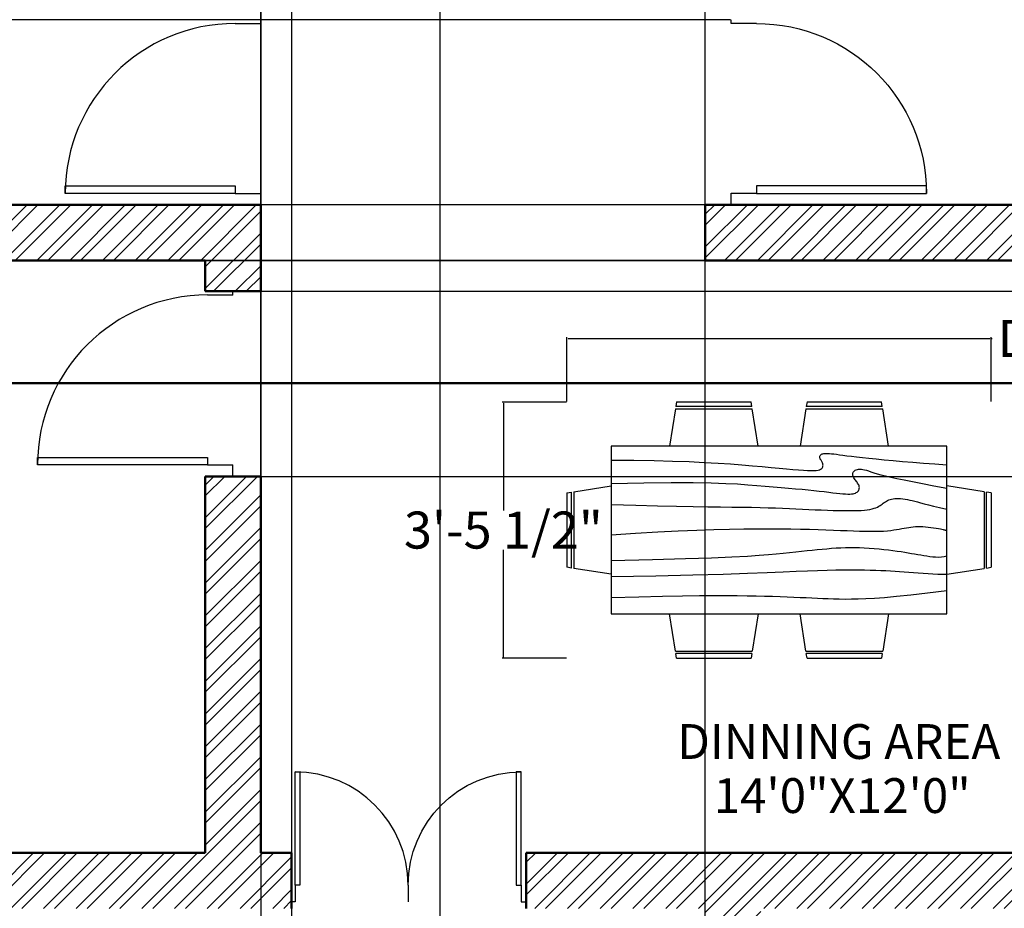
# Model space of a CAD drawing. Units: inches. Extents: x -71 to 434, y -519 to 67.
# Tile 5 of 7: x 110 to 270, y -224 to -80. Entities that reach past the tile are written whole.
import ezdxf

# ---------------------------------------------------------------- set-up
doc = ezdxf.new("R2010")
doc.units = ezdxf.units.IN
doc.header["$MEASUREMENT"] = 0
for name, color, linetype, lineweight in [('A-ANNO-DIMS', 7, 'Continuous', 18), ('A-AREA-IDEN', 7, 'Continuous', 25), ('A-WALL-PATT', 8, 'Continuous', 13), ('DOOR', 3, 'Continuous', 25), ('FURNITURE', 5, 'Continuous', 18), ('WALL', 50, 'Continuous', 50)]:
    doc.layers.add(name, color=color, linetype=linetype, lineweight=lineweight)
doc.layers.add('HATCH', color=8, linetype='Continuous')
doc.layers.add('NOI THAT', color=42, linetype='Continuous')
doc.styles.get("Standard").update_dxf_attribs({"font": 'arial.ttf'})
doc.dimstyles.get("Standard").update_dxf_attribs({"dimtxt": 6, "dimasz": 0.18, "dimexe": 0.18, "dimexo": 0.0625, "dimgap": 0.09, "dimtad": 0, "dimtih": 1, "dimtoh": 1, "dimdec": 0, "dimzin": 0, "dimdsep": 46, "dimlunit": 3, "dimtxsty": 'Standard', "dimcen": 0.09, "dimadec": 0, "dimazin": 0, "dimtfac": 1, "dimtdec": 0, "dimtofl": 0, "dimtmove": 0, "dimatfit": 3, "dimfxl": 1, "dimtolj": 1, "dimtzin": 0, "dimarcsym": 0})

# ---------------------------------------------------------------- blocks, each defined once
blk = doc.blocks.new('A$C78170A85')
at = {"layer": 'HATCH'}
for points in [[(171.5, 767.4), (258.6, 767), (337.5, 765.8), (408.9, 764), (473.5, 761.7), (532, 759), (585.1, 755.9), (633.5, 752.7), (677.8, 749.3), (718.8, 745.9), (756.5, 742.6), (790.9, 739.5), (822.2, 736.5), (850.3, 733.8), (875.4, 731.5), (897.3, 729.6), (916.3, 728.2), (932.4, 727.4), (945.8, 727.1), (956.7, 727.2), (965.6, 727.9), (972.6, 728.9), (978.1, 730.4), (982.3, 732.1), (985.5, 734.3), (988, 736.6), (989.8, 739.3), (991.1, 742.1), (991.7, 745), (991.9, 748), (991.7, 751), (991, 753.9), (990, 756.8), (988.8, 759.6), (987.3, 762.2), (985.8, 764.7), (984.2, 767.2), (982.7, 769.5), (981.4, 771.9), (980.3, 774.1), (979.5, 776.4), (979.2, 778.6), (979.2, 780.9), (979.7, 783), (980.6, 785), (982, 786.9), (983.7, 788.7), (985.9, 790.2), (988.5, 791.4), (991.6, 792.4), (995.2, 793.1), (999.4, 793.6), (1004.3, 793.7), (1010.1, 793.6), (1016.9, 793.1), (1024.7, 792.4), (1033.7, 791.4), (1043.9, 790.2), (1055.7, 788.6), (1069.2, 786.9), (1084.6, 784.9), (1102.1, 782.6), (1122, 780.2), (1144.5, 777.6), (1169.9, 774.9), (1198.1, 772), (1229.4, 769), (1263.4, 765.9), (1300.1, 762.7), (1339.4, 759.4), (1381.1, 756.1), (1425.2, 752.7), (1471.5, 749.3)], [(171.5, 677.1), (298.3, 679.7), (403.1, 680.8), (488.9, 680.7), (558.5, 679.5), (615, 677.6), (661.2, 675.2), (700.3, 672.4), (735, 669.6), (767.9, 666.8), (799.4, 664.2), (829.5, 661.7), (858.1, 659.2), (885.2, 656.9), (910.7, 654.5), (934.7, 652.3), (956.9, 650), (977.5, 647.8), (996.5, 645.6), (1013.9, 643.5), (1029.7, 641.5), (1044.1, 639.8), (1057, 638.4), (1068.6, 637.2), (1078.8, 636.5), (1087.8, 636.1), (1095.6, 636.2), (1102.4, 636.6), (1108.2, 637.4), (1113.1, 638.6), (1117.3, 640.1), (1120.9, 641.9), (1124, 644), (1126.6, 646.4), (1128.7, 649), (1130.4, 651.9), (1131.7, 654.9), (1132.4, 658.1), (1132.6, 661.3), (1132.3, 664.7), (1131.5, 668.1), (1130.1, 671.4), (1128.2, 674.8), (1126, 678.2), (1123.6, 681.6), (1121, 685), (1118.4, 688.4), (1115.8, 691.8), (1113.4, 695.1), (1111.3, 698.5), (1109.5, 701.9), (1108.2, 705.2), (1107.2, 708.5), (1106.8, 711.7), (1106.9, 714.8), (1107.6, 717.8), (1108.9, 720.7), (1110.9, 723.5), (1113.6, 726), (1116.9, 728.2), (1120.8, 730.1), (1125.1, 731.6), (1129.9, 732.6), (1135, 733), (1140.5, 732.8), (1146.3, 731.8), (1152.7, 730.3), (1159.9, 728.2), (1168.1, 725.5), (1177.6, 722.4), (1188.6, 718.9), (1201.5, 715.1), (1216.5, 710.9), (1233.8, 706.6), (1254.1, 701.9), (1277.9, 696.7), (1305.9, 690.9), (1338.7, 684.4), (1376.8, 677), (1420.9, 668.6), (1471.5, 659)], [(171.5, 595.8), (266.9, 592.9), (350.8, 590.6), (424.4, 588.9), (488.8, 587.7), (545.3, 586.9), (594.9, 586.3), (639, 585.8), (678.6, 585.3), (714.8, 584.7), (748.2, 583.9), (779.2, 583.1), (808.2, 582.1), (835.5, 581.1), (861.6, 580), (886.9, 578.9), (911.8, 577.8), (936.6, 576.7), (961.2, 575.6), (985.3, 574.6), (1008.9, 573.6), (1031.5, 572.9), (1053.1, 572.3), (1073.5, 571.9), (1092.4, 571.8), (1109.6, 571.9), (1125.2, 572.3), (1139.3, 573), (1152, 574), (1163.3, 575.3), (1173.4, 576.8), (1182.3, 578.7), (1190.2, 580.8), (1197, 583.2), (1203, 585.8), (1208.4, 588.6), (1213.1, 591.5), (1217.4, 594.5), (1221.5, 597.5), (1225.4, 600.5), (1229.3, 603.4), (1233.3, 606.1), (1237.5, 608.7), (1242, 611), (1246.8, 613.1), (1251.9, 615), (1257.4, 616.5), (1263.4, 617.6), (1269.9, 618.4), (1277, 618.8), (1284.5, 618.7), (1292.5, 618.3), (1300.9, 617.5), (1309.7, 616.3), (1318.8, 614.8), (1328.1, 613), (1337.6, 610.9), (1347.4, 608.5), (1357.9, 605.7), (1369.8, 602.5), (1383.7, 598.8), (1400.2, 594.6), (1419.9, 589.7), (1443.5, 584.1), (1471.5, 577.8)], [(171.5, 478.5), (265.6, 484.6), (351.7, 489.6), (430.6, 493.6), (502.7, 496.6), (568.7, 498.8), (629.2, 500.4), (684.7, 501.3), (735.8, 501.8), (783, 501.9), (826.7, 501.7), (867.2, 501.3), (904.8, 500.6), (939.8, 499.7), (972.5, 498.7), (1003.2, 497.6), (1032.2, 496.5), (1059.7, 495.4), (1085.8, 494.3), (1110.4, 493.4), (1133.6, 492.6), (1155.2, 492), (1175.4, 491.7), (1194.1, 491.7), (1211.2, 492), (1226.8, 492.8), (1241.1, 493.9), (1254, 495.3), (1266, 496.9), (1277, 498.7), (1287.2, 500.5), (1296.8, 502.3), (1306, 504.1), (1314.9, 505.7), (1323.7, 507.1), (1332.3, 508.3), (1341, 509.3), (1349.8, 510), (1358.9, 510.4), (1368.3, 510.4), (1378.2, 510.1), (1388.6, 509.3), (1399.3, 508.2), (1409.9, 506.9), (1420.3, 505.4), (1430, 503.8), (1438.9, 502.2), (1446.5, 500.8), (1452.7, 499.5), (1457.3, 498.5), (1460.4, 497.8), (1462.6, 497.3), (1464.1, 496.9), (1465.4, 496.7), (1466.8, 496.6), (1468.7, 496.5), (1471.5, 496.5)], [(171.5, 379.2), (330.7, 382.5), (458.9, 385.9), (560.3, 389.2), (639, 392.5), (699.2, 395.7), (745, 398.8), (780.7, 401.9), (810.2, 404.7), (837.3, 407.5), (862.5, 410.1), (886.3, 412.6), (908.7, 414.9), (929.9, 417.1), (950.2, 419.1), (969.7, 421), (988.5, 422.8), (1007, 424.4), (1025.1, 425.9), (1043, 427.1), (1060.8, 428.1), (1078.6, 428.8), (1096.5, 429.1), (1114.6, 429.2), (1133, 428.8), (1151.8, 428.1), (1170.8, 426.9), (1189.9, 425.5), (1208.8, 423.7), (1227.3, 421.8), (1245.3, 419.7), (1262.6, 417.5), (1278.9, 415.3), (1294.2, 413), (1308.5, 410.8), (1321.9, 408.5), (1334.7, 406.3), (1346.9, 404.2), (1358.8, 402.1), (1370.4, 400), (1382, 398), (1393.6, 396.1), (1405.2, 394.4), (1416.7, 393), (1428.2, 392.2), (1439.4, 392.1), (1450.5, 392.8), (1461.2, 394.4), (1471.5, 397.2)], [(171.5, 316), (344.8, 319.3), (488.1, 322.7), (605.2, 325.9), (699.8, 328.9), (776, 331.8), (837.4, 334.4), (887.9, 336.6), (931.4, 338.5), (971, 340), (1007.5, 341.1), (1041.3, 341.9), (1072.4, 342.3), (1101.2, 342.5), (1127.7, 342.4), (1152.3, 342), (1175.1, 341.6), (1196.4, 340.9), (1216.4, 340.2), (1235.3, 339.3), (1253.5, 338.3), (1271.3, 337.2), (1288.7, 335.9), (1306.3, 334.6), (1324.1, 333.3), (1342.4, 331.8), (1361.1, 330.4), (1380, 329), (1398.9, 327.7), (1417.7, 326.6), (1436.2, 325.8), (1454.2, 325.2), (1471.5, 325)], [(171.5, 234.7), (278.3, 237.7), (369.5, 239.9), (447.2, 241.5), (513.2, 242.4), (569.3, 242.9), (617.5, 243), (659.5, 242.7), (697.4, 242.2), (732.7, 241.6), (765.7, 240.9), (796.8, 240), (825.9, 239), (853.4, 238), (879.3, 237), (903.7, 235.8), (926.9, 234.7), (948.9, 233.6), (970.2, 232.5), (991.1, 231.5), (1012, 230.7), (1033.1, 230), (1055, 229.5), (1077.9, 229.3), (1102.1, 229.5), (1128.4, 230), (1157.6, 231), (1191.3, 232.9), (1230.7, 235.8), (1277.1, 239.9), (1331.8, 245.4), (1396.2, 252.7), (1471.5, 261.8)]]:
    blk.add_lwpolyline(points, dxfattribs=at)
at = {"layer": 'NOI THAT'}
for p, q in [((424.3, 993.1), (421.5, 975)), ((424.3, 993.1), (713.2, 993.1)), ((716, 975), (713.2, 993.1)), ((929.9, 993.1), (927, 975)), ((929.9, 993.1), (1218.8, 993.1)), ((1221.6, 975), (1218.8, 993.1)), ((420.1, 966), (397.5, 821.5)), ((420.1, 966), (717.5, 966)), ((716.1, 975), (421.5, 975)), ((740, 821.5), (717.4, 966)), ((925.6, 966), (903.1, 821.5)), ((925.7, 966), (1223.1, 966)), ((1221.6, 975), (927.1, 975)), ((1245.6, 821.5), (1223, 966)), ((1471.5, 821.5), (171.5, 821.5)), ((171.5, 821.5), (171.5, 171.5)), ((1471.5, 171.5), (1471.5, 821.5)), ((27.1, 645.2), (171.6, 667.8)), ((1616, 645.2), (1471.5, 667.8)), ((0, 641), (18, 643.8)), ((0, 641), (0, 352.1)), ((18.1, 349.2), (18.1, 643.7)), ((27.1, 645.1), (27.1, 347.8)), ((1616, 645.1), (1616, 347.8)), ((1643.1, 641), (1625, 643.8)), ((1625, 349.2), (1625, 643.7)), ((1643.1, 641), (1643.1, 352.1)), ((18.1, 349.3), (0, 352.1)), ((171.6, 325.3), (27.1, 347.8)), ((1471.5, 325.3), (1616, 347.8)), ((1625, 349.3), (1643.1, 352.1)), ((420.1, 27.1), (397.5, 171.6)), ((740, 171.6), (717.4, 27.1)), ((925.6, 27.1), (903.1, 171.6)), ((1245.6, 171.6), (1223, 27.1)), ((420.1, 27.1), (717.5, 27.1)), ((716.1, 18.1), (421.5, 18.1)), ((424.3, 0), (421.5, 18)), ((424.3, 0), (713.2, 0)), ((716, 18.1), (713.2, 0)), ((925.7, 27.1), (1223.1, 27.1)), ((929.9, 0), (927, 18)), ((1221.6, 18.1), (927.1, 18.1)), ((929.9, 0), (1218.8, 0)), ((1221.6, 18.1), (1218.8, 0))]:
    blk.add_line(p, q, dxfattribs=at)
at = {"layer": 'NOI THAT', "ltscale": 20}
blk.add_line((171.5, 171.5), (1471.5, 171.5), dxfattribs=at)
blk = doc.blocks.new('*U13')
for p, q in [((0, 0), (0, -6)), ((40, 0), (40, -6))]:
    blk.add_line(p, q)
blk.add_lwpolyline([(0, 0), (0, 40), (1.75, 40), (1.75, 0)], close=True)
blk.add_arc((0, 0), 40, 0, 90)
blk = doc.blocks.new('*D42')
at = {"layer": 'A-ANNO-DIMS', "color": 0, "lineweight": -2, "transparency": 16777216}
for p, q in [((199.01, -142.05), (199.01, -131.63)), ((199.19, -131.81), (267.52, -131.81)), ((267.7, -142.05), (267.7, -131.63)), ((267.7, -131.81), (267.88, -131.81))]:
    blk.add_line(p, q, dxfattribs=at)
at = {"layer": 'A-ANNO-DIMS', "color": 0, "transparency": 16777216}
for points in [[(199.19, -131.78), (199.19, -131.84), (199.01, -131.81)], [(267.52, -131.78), (267.52, -131.84), (267.7, -131.81)]]:
    blk.add_solid(points, dxfattribs=at)
at = {"layer": 'Defpoints', "color": 0, "transparency": 16777216}
for p in [(267.7, -131.81), (199.01, -142.12), (267.7, -142.12)]:
    blk.add_point(p, dxfattribs=at)
at = {"layer": 'A-ANNO-DIMS', "color": 0, "transparency": 16777216, "insert": (307.94, -131.81), "char_height": 6, "attachment_point": 5}
blk.add_mtext('\\A1;DINING SET 5\'-8 1/2"', dxfattribs=at)
blk = doc.blocks.new('*D43')
at = {"layer": 'A-ANNO-DIMS', "color": 0, "lineweight": -2, "transparency": 16777216}
for p, q in [((198.95, -142.12), (188.53, -142.12)), ((188.71, -142.3), (188.71, -159.68)), ((188.71, -183.45), (188.71, -166.07)), ((198.95, -183.63), (188.53, -183.63))]:
    blk.add_line(p, q, dxfattribs=at)
at = {"layer": 'A-ANNO-DIMS', "color": 0, "transparency": 16777216}
for points in [[(188.68, -142.3), (188.74, -142.3), (188.71, -142.12)], [(188.68, -183.45), (188.74, -183.45), (188.71, -183.63)]]:
    blk.add_solid(points, dxfattribs=at)
at = {"layer": 'Defpoints', "color": 0, "transparency": 16777216}
for p in [(188.71, -142.12), (199.01, -142.12), (199.01, -183.63)]:
    blk.add_point(p, dxfattribs=at)
at = {"layer": 'A-ANNO-DIMS', "color": 0, "transparency": 16777216, "insert": (188.71, -162.87), "char_height": 6, "attachment_point": 5}
blk.add_mtext('\\A1;3\'-5 1/2"', dxfattribs=at)
blk = doc.blocks.new('*D49')
at = {"layer": 'A-ANNO-DIMS', "color": 0, "lineweight": -2, "transparency": 16777216}
for p, q in [((221.41, -473.1), (221.41, 58.56)), ((221.59, 58.38), (262.84, 58.38)), ((320.23, 58.38), (278.98, 58.38)), ((320.41, -473.1), (320.41, 58.56))]:
    blk.add_line(p, q, dxfattribs=at)
at = {"layer": 'A-ANNO-DIMS', "color": 0, "transparency": 16777216}
for points in [[(221.59, 58.41), (221.59, 58.35), (221.41, 58.38)], [(320.23, 58.41), (320.23, 58.35), (320.41, 58.38)]]:
    blk.add_solid(points, dxfattribs=at)
at = {"layer": 'Defpoints', "color": 0, "transparency": 16777216}
for p in [(320.41, 58.38), (221.41, -473.17), (320.41, -473.17)]:
    blk.add_point(p, dxfattribs=at)
at = {"layer": 'A-ANNO-DIMS', "color": 0, "transparency": 16777216, "insert": (270.91, 58.38), "char_height": 6, "attachment_point": 5}
blk.add_mtext('\\A1;8\'-3"', dxfattribs=at)
blk = doc.blocks.new('*D56')
at = {"layer": 'A-ANNO-DIMS', "color": 0, "lineweight": -2, "transparency": 16777216}
for p, q in [((154.41, -71.23), (154.41, -509.9)), ((178.41, -71.23), (178.41, -509.9)), ((154.59, -509.72), (158.29, -509.72)), ((178.23, -509.72), (174.52, -509.72))]:
    blk.add_line(p, q, dxfattribs=at)
at = {"layer": 'A-ANNO-DIMS', "color": 0, "transparency": 16777216}
for points in [[(154.59, -509.69), (154.59, -509.75), (154.41, -509.72)], [(178.23, -509.69), (178.23, -509.75), (178.41, -509.72)]]:
    blk.add_solid(points, dxfattribs=at)
at = {"layer": 'Defpoints', "color": 0, "transparency": 16777216}
for p in [(154.41, -71.17), (178.41, -71.17), (178.41, -509.72)]:
    blk.add_point(p, dxfattribs=at)
at = {"layer": 'A-ANNO-DIMS', "color": 0, "transparency": 16777216, "insert": (166.41, -509.72), "char_height": 6, "attachment_point": 5}
blk.add_mtext('\\A1;2\'-0"', dxfattribs=at)
blk = doc.blocks.new('*D57')
at = {"layer": 'A-ANNO-DIMS', "color": 0, "lineweight": -2, "transparency": 16777216}
for p, q in [((149.47, -124.17), (411.14, -124.17)), ((410.96, -124.35), (410.96, -136.01)), ((410.96, -153.99), (410.96, -142.32)), ((149.47, -154.17), (411.14, -154.17))]:
    blk.add_line(p, q, dxfattribs=at)
at = {"layer": 'A-ANNO-DIMS', "color": 0, "transparency": 16777216}
for points in [[(410.93, -124.35), (410.99, -124.35), (410.96, -124.17)], [(410.93, -153.99), (410.99, -153.99), (410.96, -154.17)]]:
    blk.add_solid(points, dxfattribs=at)
at = {"layer": 'Defpoints', "color": 0, "transparency": 16777216}
for p in [(149.41, -124.17), (149.41, -154.17), (410.96, -154.17)]:
    blk.add_point(p, dxfattribs=at)
at = {"layer": 'A-ANNO-DIMS', "color": 0, "transparency": 16777216, "insert": (410.96, -139.17), "char_height": 6, "attachment_point": 5}
blk.add_mtext('\\A1;2\'-6"', dxfattribs=at)
blk = doc.blocks.new('*D59')
at = {"layer": 'A-ANNO-DIMS', "color": 0, "lineweight": -2, "transparency": 16777216}
for p, q in [((149.35, -80.17), (-40.32, -80.17)), ((-40.14, -80.35), (-40.14, -92.01)), ((-40.14, -109.99), (-40.14, -98.32)), ((149.35, -110.17), (-40.32, -110.17))]:
    blk.add_line(p, q, dxfattribs=at)
at = {"layer": 'A-ANNO-DIMS', "color": 0, "transparency": 16777216}
for points in [[(-40.17, -80.35), (-40.11, -80.35), (-40.14, -80.17)], [(-40.17, -109.99), (-40.11, -109.99), (-40.14, -110.17)]]:
    blk.add_solid(points, dxfattribs=at)
at = {"layer": 'Defpoints', "color": 0, "transparency": 16777216}
for p in [(149.41, -80.17), (-40.14, -110.17), (149.41, -110.17)]:
    blk.add_point(p, dxfattribs=at)
at = {"layer": 'A-ANNO-DIMS', "color": 0, "transparency": 16777216, "insert": (-40.14, -95.17), "char_height": 6, "attachment_point": 5}
blk.add_mtext('\\A1;2\'-6"', dxfattribs=at)
blk = doc.blocks.new('*D62')
at = {"layer": 'A-ANNO-DIMS', "color": 0, "lineweight": -2, "transparency": 16777216}
for p, q in [((149.41, -71.23), (149.41, -509.9)), ((154.41, -71.23), (154.41, -509.9)), ((149.59, -509.72), (154.23, -509.72)), ((154.41, -509.72), (154.59, -509.72))]:
    blk.add_line(p, q, dxfattribs=at)
at = {"layer": 'A-ANNO-DIMS', "color": 0, "transparency": 16777216}
for points in [[(149.59, -509.69), (149.59, -509.75), (149.41, -509.72)], [(154.23, -509.69), (154.23, -509.75), (154.41, -509.72)]]:
    blk.add_solid(points, dxfattribs=at)
at = {"layer": 'Defpoints', "color": 0, "transparency": 16777216}
for p in [(149.41, -71.17), (154.41, -71.17), (154.41, -509.72)]:
    blk.add_point(p, dxfattribs=at)
at = {"layer": 'A-ANNO-DIMS', "color": 0, "transparency": 16777216, "insert": (162.65, -509.72), "char_height": 6, "attachment_point": 5}
blk.add_mtext('\\A1;0\'-5"', dxfattribs=at)
blk = doc.blocks.new('*D64')
at = {"layer": 'A-ANNO-DIMS', "color": 0, "lineweight": -2, "transparency": 16777216}
for p, q in [((320.35, -119.17), (-40.32, -119.17)), ((-40.14, -119.35), (-40.14, -126)), ((-40.14, -138.97), (-40.14, -132.31)), ((320.35, -139.15), (-40.32, -139.15))]:
    blk.add_line(p, q, dxfattribs=at)
at = {"layer": 'A-ANNO-DIMS', "color": 0, "transparency": 16777216}
for points in [[(-40.17, -119.35), (-40.11, -119.35), (-40.14, -119.17)], [(-40.17, -138.97), (-40.11, -138.97), (-40.14, -139.15)]]:
    blk.add_solid(points, dxfattribs=at)
at = {"layer": 'Defpoints', "color": 0, "transparency": 16777216}
for p in [(320.41, -119.17), (-40.14, -139.15), (320.41, -139.15)]:
    blk.add_point(p, dxfattribs=at)
at = {"layer": 'A-ANNO-DIMS', "color": 0, "transparency": 16777216, "insert": (-40.14, -129.16), "char_height": 6, "attachment_point": 5}
blk.add_mtext('\\A1;1\'-8"', dxfattribs=at)
blk = doc.blocks.new('*D67')
at = {"layer": 'A-ANNO-DIMS', "color": 0, "lineweight": -2, "transparency": 16777216}
for p, q in [((107.56, -119.17), (411.14, -119.17)), ((410.96, -119.35), (410.96, -125.92)), ((410.96, -138.8), (410.96, -132.22)), ((107.56, -138.98), (411.14, -138.98))]:
    blk.add_line(p, q, dxfattribs=at)
at = {"layer": 'A-ANNO-DIMS', "color": 0, "transparency": 16777216}
for points in [[(410.93, -119.35), (410.99, -119.35), (410.96, -119.17)], [(410.93, -138.8), (410.99, -138.8), (410.96, -138.98)]]:
    blk.add_solid(points, dxfattribs=at)
at = {"layer": 'Defpoints', "color": 0, "transparency": 16777216}
for p in [(107.49, -119.17), (107.49, -138.98), (410.96, -138.98)]:
    blk.add_point(p, dxfattribs=at)
at = {"layer": 'A-ANNO-DIMS', "color": 0, "transparency": 16777216, "insert": (410.96, -129.07), "char_height": 6, "attachment_point": 5}
blk.add_mtext('\\A1;1\'-8"', dxfattribs=at)
blk = doc.blocks.new('*D69')
at = {"layer": 'A-ANNO-DIMS', "color": 0, "lineweight": -2, "transparency": 16777216}
for p, q in [((149.41, -215.1), (149.41, 58.56)), ((149.59, 58.38), (220.29, 58.38)), ((311.23, 58.38), (240.52, 58.38)), ((311.41, -215.1), (311.41, 58.56))]:
    blk.add_line(p, q, dxfattribs=at)
at = {"layer": 'A-ANNO-DIMS', "color": 0, "transparency": 16777216}
for points in [[(149.59, 58.41), (149.59, 58.35), (149.41, 58.38)], [(311.23, 58.41), (311.23, 58.35), (311.41, 58.38)]]:
    blk.add_solid(points, dxfattribs=at)
at = {"layer": 'Defpoints', "color": 0, "transparency": 16777216}
for p in [(311.41, 58.38), (149.41, -215.17), (311.41, -215.17)]:
    blk.add_point(p, dxfattribs=at)
at = {"layer": 'A-ANNO-DIMS', "color": 0, "transparency": 16777216, "insert": (230.41, 58.38), "char_height": 6, "attachment_point": 5}
blk.add_mtext('\\A1;13\'-6"', dxfattribs=at)
blk = doc.blocks.new('*D75')
at = {"layer": 'A-ANNO-DIMS', "color": 0, "lineweight": -2, "transparency": 16777216}
for p, q in [((225.52, -80.17), (-40.32, -80.17)), ((-40.14, -80.35), (-40.14, -92.01)), ((-40.14, -109.99), (-40.14, -98.32)), ((221.35, -110.17), (-40.32, -110.17))]:
    blk.add_line(p, q, dxfattribs=at)
at = {"layer": 'A-ANNO-DIMS', "color": 0, "transparency": 16777216}
for points in [[(-40.17, -80.35), (-40.11, -80.35), (-40.14, -80.17)], [(-40.17, -109.99), (-40.11, -109.99), (-40.14, -110.17)]]:
    blk.add_solid(points, dxfattribs=at)
at = {"layer": 'Defpoints', "color": 0, "transparency": 16777216}
for p in [(225.58, -80.17), (-40.14, -110.17), (221.41, -110.17)]:
    blk.add_point(p, dxfattribs=at)
at = {"layer": 'A-ANNO-DIMS', "color": 0, "transparency": 16777216, "insert": (-40.14, -95.17), "char_height": 6, "attachment_point": 5}
blk.add_mtext('\\A1;2\'-6"', dxfattribs=at)

msp = doc.modelspace()

# ---------------------------------------------------------------- hatches: boundary and pattern name
at = {"layer": 'A-WALL-PATT'}
h = msp.add_hatch(dxfattribs=at)
h.set_pattern_fill('ANSI32', color=256, scale=10)
h.set_pattern_definition([(45, (-213.138, 0), (-2.65165, 2.65165), []), (45, (-211.37, 0), (-2.65165, 2.65165), [])])
h.paths.add_polyline_path([(383.41, 30.83), (230.41, 30.83), (149.41, 30.83), (-12.59, 30.83), (-12.59, -20.17), (-3.59, -20.17), (-3.59, 21.83), (140.41, 21.83), (140.41, 15.83), (149.41, 15.83), (149.41, 21.83), (221.41, 21.83), (221.41, 15.83), (230.41, 15.83), (230.41, 21.83), (374.41, 21.83), (374.41, -110.17), (369.41, -110.17), (369.41, -119.17), (374.41, -119.17), (374.41, -215.17), (320.41, -215.17), (320.41, -119.17), (345.41, -119.17), (345.41, -110.17), (221.41, -110.17), (221.41, -119.17), (311.41, -119.17), (311.41, -215.17), (192.42, -215.17), (192.42, -224.17), (221.41, -224.17), (221.41, -228.23), (230.41, -228.23), (230.41, -224.17), (374.41, -224.17), (374.41, -368.17), (230.41, -368.17), (230.41, -266.34), (221.41, -266.34), (221.41, -368.17), (192.08, -368.17), (192.08, -377.17), (230.41, -377.17), (374.41, -377.17), (374.41, -473.17), (230.41, -473.17), (212.41, -473.17), (212.41, -482.17), (383.41, -482.17), (383.41, -377.17), (383.41, -224.17), (383.41, -119.17)])
h.paths.add_polyline_path([(149.41, -110.17), (-3.59, -110.17), (-3.59, -68.17), (-12.59, -68.17), (-12.59, -276.67), (-3.59, -276.67), (-3.59, -224.17), (154.41, -224.17), (154.41, -215.17), (149.41, -215.17), (149.41, -154.17), (140.41, -154.17), (140.41, -215.17), (-3.59, -215.17), (-3.59, -119.17), (19.82, -119.17), (140.41, -119.17), (140.41, -124.17), (149.41, -124.17)])
h.paths.add_polyline_path([(84.91, -368.17), (-3.59, -368.17), (-3.59, -324.67), (-12.59, -324.67), (-12.59, -377.17), (-12.59, -401.17), (-3.59, -401.17), (-3.59, -377.17), (84.91, -377.17)], flags=17)
h.paths.add_polyline_path([(1.41, -473.17), (-3.59, -473.17), (-3.59, -468.17), (-12.59, -468.17), (-12.59, -482.17), (1.41, -482.17)], flags=17)

# ---------------------------------------------------------------- linework, layer by layer
at = {"layer": 'DOOR'}
for p, q in [((149.41, -80.78), (149.41, -80.17)), ((225.58, -80.78), (225.58, -80.17)), ((149.41, -110.17), (149.41, -108.3)), ((225.58, -110.17), (225.58, -108.3)), ((144.91, -124.78), (144.91, -124.17)), ((144.91, -154.17), (144.91, -152.3)), ((154.96, -223.14), (154.41, -223.14)), ((191.6, -223.14), (192.42, -223.14))]:
    msp.add_line(p, q, dxfattribs=at)
at = {"layer": 'WALL'}
for p, q in [((-3.59, -110.17), (149.41, -110.17)), ((149.41, -124.17), (149.41, -110.17)), ((221.41, -119.17), (221.41, -110.17)), ((345.41, -110.17), (221.41, -110.17)), ((-3.59, -119.17), (140.41, -119.17)), ((140.41, -124.17), (140.41, -119.17)), ((311.41, -119.17), (221.41, -119.17)), ((140.41, -124.17), (149.41, -124.17)), ((140.41, -215.17), (140.41, -154.17)), ((140.41, -154.17), (149.41, -154.17)), ((149.41, -215.17), (149.41, -154.17)), ((-3.59, -215.17), (140.41, -215.17)), ((149.41, -215.17), (154.41, -215.17)), ((154.41, -224.17), (154.41, -215.17)), ((192.42, -224.17), (192.42, -215.17)), ((192.42, -215.17), (311.41, -215.17))]:
    msp.add_line(p, q, dxfattribs=at)

# ---------------------------------------------------------------- block references
at = {"layer": 'DOOR', "yscale": 0.6882691303572923, "zscale": 0.6882691303572923}
for p, xscale, rotation in [((145.28, -108.31), 0.6882691303572923, 90), ((229.71, -108.31), -0.6882691303572923, 270), ((140.78, -152.31), 0.6882691303572923, 90)]:
    msp.add_blockref('*U13', p, dxfattribs=dict(at, xscale=xscale, rotation=rotation))
at = {"layer": 'DOOR', "yscale": 0.4579749947461901, "zscale": 0.4579749947461901}
for p, xscale in [((154.96, -220.39), 0.4579749947461901), ((191.6, -220.39), -0.4579749947461901)]:
    msp.add_blockref('*U13', p, dxfattribs=dict(at, xscale=xscale))
at = {"layer": 'FURNITURE', "xscale": 0.0418072086103679, "yscale": 0.0418072086103679, "zscale": 0.0418072086103679}
msp.add_blockref('A$C78170A85', (199.01, -183.63), dxfattribs=at)

# ---------------------------------------------------------------- texts
at = {"layer": 'A-AREA-IDEN'}
for s, p in [('DINNING AREA', (216.87, -199.96)), ('14\'0"X12\'0"', (222.77, -208.72))]:
    msp.add_text(s, height=5.6432, dxfattribs=at).set_placement(p)

# ---------------------------------------------------------------- dimensions: what is measured, and where the dimension line sits
at = {"layer": 'A-ANNO-DIMS'}
for base, p1, p2, picture, middle in [((311.41, 58.38), (149.41, -215.17), (311.41, -215.17), '*D69', (230.41, 58.38)), ((320.41, 58.38), (221.41, -473.17), (320.41, -473.17), '*D49', (270.91, 58.38)), ((154.41, -509.72), (149.41, -71.17), (154.41, -71.17), '*D62', (162.65, -509.72)), ((178.41, -509.72), (154.41, -71.17), (178.41, -71.17), '*D56', (166.41, -509.72))]:
    dim = msp.add_linear_dim(base=base, p1=p1, p2=p2, dimstyle='Standard', override={"dimdec": 1, "dimlfac": 1, "dimrnd": 0, "dimzin": 1, "dimdsep": 46, "dimlunit": 4, "dimfrac": 2}, dxfattribs=at)
    dim.commit()
    dim.dimension.update_dxf_attribs({"geometry": picture, "text_midpoint": middle})
for base, p1, p2, picture, middle in [((-40.14, -110.17), (149.41, -80.17), (149.41, -110.17), '*D59', (-40.14, -95.17)), ((-40.14, -110.17), (225.58, -80.17), (221.41, -110.17), '*D75', (-40.14, -95.17)), ((-40.14, -139.15), (320.41, -119.17), (320.41, -139.15), '*D64', (-40.14, -129.16)), ((410.96, -138.98), (107.49, -119.17), (107.49, -138.98), '*D67', (410.96, -129.07)), ((410.96, -154.17), (149.41, -124.17), (149.41, -154.17), '*D57', (410.96, -139.17)), ((188.71, -142.12), (199.01, -183.63), (199.01, -142.12), '*D43', (188.71, -162.87))]:
    dim = msp.add_linear_dim(base=base, p1=p1, p2=p2, angle=90, dimstyle='Standard', override={"dimdec": 1, "dimlfac": 1, "dimrnd": 0, "dimzin": 1, "dimdsep": 46, "dimlunit": 4, "dimfrac": 2}, dxfattribs=at)
    dim.commit()
    dim.dimension.update_dxf_attribs({"geometry": picture, "text_midpoint": middle})
dim = msp.add_linear_dim(base=(267.7, -131.81), p1=(199.01, -142.12), p2=(267.7, -142.12), text='DINING SET <>', dimstyle='Standard', override={"dimdec": 1, "dimlfac": 1, "dimrnd": 0, "dimzin": 1, "dimdsep": 46, "dimlunit": 4, "dimfrac": 2}, dxfattribs=at)
dim.commit()
dim.dimension.update_dxf_attribs({"geometry": '*D42', "text_midpoint": (307.94, -131.81)})

doc.saveas('drawing.dxf')
